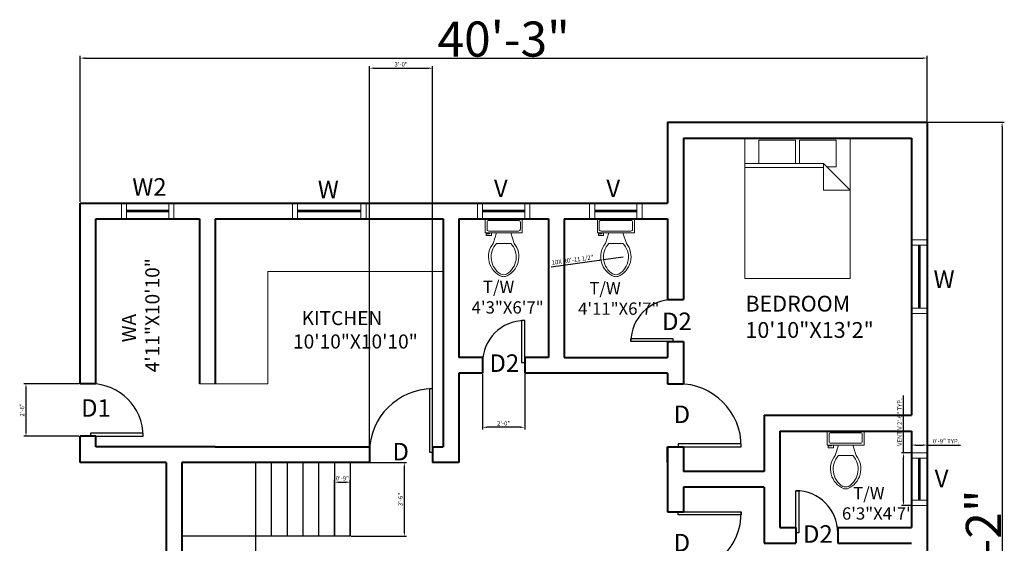
# Model space of a CAD drawing. Units: inches. Extents: x 4878 to 9282, y 5367 to 6617.
# Tile 11 of 14: x 7961 to 8522, y 6318 to 6616. Entities that reach past the tile are written whole.
import ezdxf

# ---------------------------------------------------------------- set-up
doc = ezdxf.new("R2010")
doc.units = ezdxf.units.IN
for name, color, linetype, lineweight in [('A-ANNO-DIMS', 2, 'Continuous', 18), ('A-ANNO-TEXT', 7, 'Continuous', 18), ('A-AREA-IDEN', 4, 'Continuous', 18), ('A-DOOR', 3, 'Continuous', 25), ('A-FLOR-FIXT', 9, 'Continuous', 20), ('A-FLOR-STRS', 7, 'Continuous', 25), ('A-FURN', 8, 'Continuous', 18), ('A-GLAZ', 30, 'Continuous', 20), ('A-WALL', 7, 'Continuous', 40)]:
    doc.layers.add(name, color=color, linetype=linetype, lineweight=lineweight)
doc.styles.get("Standard").update_dxf_attribs({"font": 'arial.ttf'})
doc.dimstyles.new('ISO-25', dxfattribs={"dimtxt": 2.5, "dimasz": 2.5, "dimexe": 1.25, "dimexo": 0.625, "dimtad": 1, "dimdec": 0, "dimlunit": 3, "dimtxsty": 'Standard', "dimcen": 2.5, "dimadec": 0, "dimazin": 0, "dimtfac": 1, "dimtdec": 0, "dimtmove": 0, "dimatfit": 3, "dimfxl": 1, "dimarcsym": 0})

# ---------------------------------------------------------------- blocks, each defined once
blk = doc.blocks.new('Toilet - top')
for p, q in [((9.5, -6), (9.5, -2)), ((-10, -8.5), (-8, -8.5)), ((-10, -9.5), (-10, -8.5)), ((-7, -9.5), (-10, -9.5)), ((-8, -8.5), (-8, -8)), ((-7, -8), (-7, -9.5)), ((-4, -8), (-6, -14)), ((4, -8), (6, -14)), ((4, -14), (-4, -14))]:
    blk.add_line(p, q)
blk.add_lwpolyline([(10.5, -8), (10.5, 0), (-10.5, 0), (-10.5, -8)], close=True)
for points in [[(-9.5, -2), (-9.5, -6)], [(8.5, -1), (-8.5, -1)], [(-8.5, -7), (8.5, -7)]]:
    blk.add_lwpolyline(points)
for centre, radius, start, end in [((-8.62, -1.88), 0.884, 81.8699, 188.1301), ((8.62, -1.88), 0.884, 351.8699, 98.1301), ((-8.62, -6.12), 0.884, 171.8699, 278.1301), ((8.62, -6.12), 0.884, 261.8699, 8.1301), ((3.52, -21.58), 12.17, 141.4691, 247.9714), ((4.2, -21.82), 11.33, 136.3677, 238.9468), ((-3.52, -21.58), 12.17, 292.0284, 38.5307), ((-4.2, -21.82), 11.33, 301.053, 43.6321), ((0, -27.88), 4, 245.7318, 294.2682), ((0, -29), 4, 254.8605, 285.1395)]:
    blk.add_arc(centre, radius, start, end)
blk = doc.blocks.new('Bed - Queen')
for p, q in [((0, -80.00003), (0, 0)), ((0, 0), (59.99999, 0)), ((59.99999, 0), (59.99999, -80.00003)), ((7.99999, -1.2), (28.79998, -1.2)), ((7.99999, -14.4), (7.99999, -1.2)), ((28.79998, -1.2), (28.79998, -14.4)), ((31.19999, -1.2), (51.99999, -1.2)), ((31.19999, -14.4), (31.19999, -1.2)), ((51.99999, -1.2), (51.99999, -16.4)), ((0, -14.4), (44.8, -14.4)), ((44.8, -16.8), (0, -16.8)), ((59.99999, -29.6), (44.8, -14.4)), ((44.8, -14.4), (44.8, -29.6)), ((51.99999, -16.4), (46.79936, -16.4)), ((44.8, -29.6), (59.99999, -29.6)), ((59.99999, -80.00003), (0, -80.00003))]:
    blk.add_line(p, q)
blk = doc.blocks.new('*U19')
for p, q in [((0, 0), (0, -6)), ((-36, 0), (-36, -6))]:
    blk.add_line(p, q)
blk.add_lwpolyline([(0, 0), (0, 36), (-1.75, 36), (-1.75, 0)], close=True)
blk.add_arc((0, 0), 36, 90, 180)
blk = doc.blocks.new('*U21')
for p, q in [((-24, 0), (-24, -6)), ((0, 0), (0, -6))]:
    blk.add_line(p, q)
blk.add_lwpolyline([(0, 0), (0, 24), (-1.75, 24), (-1.75, 0)], close=True)
blk.add_arc((0, 0), 24, 90, 180)
blk = doc.blocks.new('*U22')
for p, q in [((0, 0), (0, -6)), ((24, 0), (24, -6))]:
    blk.add_line(p, q)
blk.add_lwpolyline([(0, 0), (0, 24), (1.75, 24), (1.75, 0)], close=True)
blk.add_arc((0, 0), 24, 0, 90)
blk = doc.blocks.new('*U20')
for p, q in [((-36, 0), (-36, 6)), ((0, 0), (0, 6))]:
    blk.add_line(p, q)
blk.add_lwpolyline([(0, 0), (0, -36), (-1.75, -36), (-1.75, 0)], close=True)
blk.add_arc((0, 0), 36, 180, 270)
blk = doc.blocks.new('*U23')
for p, q in [((0, 0), (0, 6)), ((36, 0), (36, 6))]:
    blk.add_line(p, q)
blk.add_lwpolyline([(0, 0), (0, -36), (1.75, -36), (1.75, 0)], close=True)
blk.add_arc((0, 0), 36, 270, 360)
blk = doc.blocks.new('*U24')
for p, q in [((0, 0), (0, 6)), ((30, 0), (30, 6))]:
    blk.add_line(p, q)
blk.add_lwpolyline([(0, 0), (0, -30), (1.75, -30), (1.75, 0)], close=True)
blk.add_arc((0, 0), 30, 270, 360)
blk = doc.blocks.new('*U25')
for p, q in [((0, 0), (0, -6)), ((24, 0), (24, -6))]:
    blk.add_line(p, q)
blk.add_lwpolyline([(0, 0), (0, 24), (1.75, 24), (1.75, 0)], close=True)
blk.add_arc((0, 0), 24, 0, 90)
blk = doc.blocks.new('*D26')
at = {"layer": 'A-ANNO-DIMS', "color": 0, "lineweight": -2, "transparency": 16777216}
for p, q in [((8478.72, 6557.77), (8522.05, 6557.77)), ((8520.8, 6555.27), (8520.8, 6066.27)), ((8478.72, 6063.77), (8522.05, 6063.77))]:
    blk.add_line(p, q, dxfattribs=at)
at = {"layer": 'A-ANNO-DIMS', "color": 0, "transparency": 16777216}
for points in [[(8520.39, 6555.27), (8521.22, 6555.27), (8520.8, 6557.77)], [(8520.39, 6066.27), (8521.22, 6066.27), (8520.8, 6063.77)]]:
    blk.add_solid(points, dxfattribs=at)
at = {"layer": 'Defpoints', "color": 0, "transparency": 16777216}
for p in [(8478.1, 6557.77), (8478.1, 6063.77), (8520.8, 6063.77)]:
    blk.add_point(p, dxfattribs=at)
at = {"layer": 'A-ANNO-DIMS', "color": 0, "transparency": 16777216, "insert": (8510.14, 6310.77), "char_height": 2.5, "attachment_point": 5, "rotation": 90}
blk.add_mtext('{\\H8x;41\'-2"}', dxfattribs=at)
blk = doc.blocks.new('*D27')
at = {"layer": 'A-ANNO-DIMS', "color": 0, "lineweight": -2, "transparency": 16777216}
for p, q in [((7995.1, 6512.4), (7995.1, 6595.64)), ((7997.6, 6594.39), (8475.6, 6594.39)), ((8478.1, 6512.4), (8478.1, 6595.64))]:
    blk.add_line(p, q, dxfattribs=at)
at = {"layer": 'A-ANNO-DIMS', "color": 0, "transparency": 16777216}
for points in [[(7997.6, 6594.81), (7997.6, 6593.97), (7995.1, 6594.39)], [(8475.6, 6594.81), (8475.6, 6593.97), (8478.1, 6594.39)]]:
    blk.add_solid(points, dxfattribs=at)
at = {"layer": 'Defpoints', "color": 0, "transparency": 16777216}
for p in [(8478.1, 6594.39), (7995.1, 6511.77), (8478.1, 6511.77)]:
    blk.add_point(p, dxfattribs=at)
at = {"layer": 'A-ANNO-DIMS', "color": 0, "transparency": 16777216, "insert": (8236.6, 6605.23), "char_height": 2.5, "attachment_point": 5}
blk.add_mtext('{\\H8x;40\'-3"}', dxfattribs=at)
blk = doc.blocks.new('WINDOW-PLAN-36IN')
for p, q in [((0, 0), (0, 9)), ((3, 0), (3, 9)), ((39, 0), (39, 9)), ((42, 0), (42, 9)), ((3, 5), (39, 5)), ((3, 4.5), (39, 4.5)), ((3, 4), (39, 4))]:
    blk.add_line(p, q)
blk = doc.blocks.new('WINDOW-PLAN-24IN')
for p, q in [((9, 30), (0, 30)), ((9, 27), (0, 27)), ((4, 3), (4, 27)), ((4.5, 3), (4.5, 27)), ((5, 3), (5, 27)), ((9, 3), (0, 3)), ((9, 0), (0, 0))]:
    blk.add_line(p, q)
blk = doc.blocks.new('*D41')
at = {"layer": 'A-ANNO-DIMS', "color": 0, "lineweight": -2, "transparency": 16777216}
for p, q in [((8464.6, 6369.27), (8464.6, 6401.97)), ((8468.47, 6369.27), (8463.35, 6369.27)), ((8464.6, 6341.77), (8464.6, 6366.77)), ((8468.47, 6339.27), (8463.35, 6339.27))]:
    blk.add_line(p, q, dxfattribs=at)
at = {"layer": 'A-ANNO-DIMS', "color": 0, "transparency": 16777216}
for points in [[(8464.18, 6366.77), (8465.01, 6366.77), (8464.6, 6369.27)], [(8464.18, 6341.77), (8465.01, 6341.77), (8464.6, 6339.27)]]:
    blk.add_solid(points, dxfattribs=at)
at = {"layer": 'Defpoints', "color": 0, "transparency": 16777216}
for p in [(8464.6, 6369.27), (8469.1, 6369.27), (8469.1, 6339.27)]:
    blk.add_point(p, dxfattribs=at)
at = {"layer": 'A-ANNO-DIMS', "color": 0, "transparency": 16777216, "insert": (8462.69, 6386.87), "char_height": 2.5, "attachment_point": 5, "rotation": 90}
blk.add_mtext('VENT V 2\'-6" TYP.', dxfattribs=at)
blk = doc.blocks.new('*D42')
at = {"layer": 'A-ANNO-DIMS', "color": 0, "lineweight": -2, "transparency": 16777216}
for p, q in [((8469.1, 6369.9), (8469.1, 6375.02)), ((8471.6, 6373.77), (8475.6, 6373.77)), ((8478.1, 6369.9), (8478.1, 6375.02)), ((8478.1, 6373.77), (8497.08, 6373.77))]:
    blk.add_line(p, q, dxfattribs=at)
at = {"layer": 'A-ANNO-DIMS', "color": 0, "transparency": 16777216}
for points in [[(8471.6, 6374.19), (8471.6, 6373.35), (8469.1, 6373.77)], [(8475.6, 6374.19), (8475.6, 6373.35), (8478.1, 6373.77)]]:
    blk.add_solid(points, dxfattribs=at)
at = {"layer": 'Defpoints', "color": 0, "transparency": 16777216}
for p in [(8478.1, 6373.77), (8469.1, 6369.27), (8478.1, 6369.27)]:
    blk.add_point(p, dxfattribs=at)
at = {"layer": 'A-ANNO-DIMS', "color": 0, "transparency": 16777216, "insert": (8488.84, 6375.67), "char_height": 2.5, "attachment_point": 5}
blk.add_mtext('0\'-9" TYP.', dxfattribs=at)
blk = doc.blocks.new('*D107')
at = {"layer": 'A-ANNO-DIMS', "color": 0, "lineweight": -2, "transparency": 16777216}
for p, q in [((7994.47, 6408.77), (7963, 6408.77)), ((7964.25, 6381.27), (7964.25, 6406.27)), ((7994.47, 6378.77), (7963, 6378.77))]:
    blk.add_line(p, q, dxfattribs=at)
at = {"layer": 'A-ANNO-DIMS', "color": 0, "transparency": 16777216}
for points in [[(7963.83, 6406.27), (7964.66, 6406.27), (7964.25, 6408.77)], [(7963.83, 6381.27), (7964.66, 6381.27), (7964.25, 6378.77)]]:
    blk.add_solid(points, dxfattribs=at)
at = {"layer": 'Defpoints', "color": 0, "transparency": 16777216}
for p in [(7964.25, 6408.77), (7995.1, 6408.77), (7995.1, 6378.77)]:
    blk.add_point(p, dxfattribs=at)
at = {"layer": 'A-ANNO-DIMS', "color": 0, "transparency": 16777216, "insert": (7962.34, 6393.77), "char_height": 2.5, "attachment_point": 5, "rotation": 90}
blk.add_mtext('2\'-6"', dxfattribs=at)
blk = doc.blocks.new('*D108')
at = {"layer": 'A-ANNO-DIMS', "color": 0, "lineweight": -2, "transparency": 16777216}
for p, q in [((8160.1, 6373.4), (8160.1, 6589.87)), ((8162.6, 6588.62), (8193.6, 6588.62)), ((8196.1, 6373.4), (8196.1, 6589.87))]:
    blk.add_line(p, q, dxfattribs=at)
at = {"layer": 'A-ANNO-DIMS', "color": 0, "transparency": 16777216}
for points in [[(8162.6, 6589.04), (8162.6, 6588.2), (8160.1, 6588.62)], [(8193.6, 6589.04), (8193.6, 6588.2), (8196.1, 6588.62)]]:
    blk.add_solid(points, dxfattribs=at)
at = {"layer": 'Defpoints', "color": 0, "transparency": 16777216}
for p in [(8196.1, 6588.62), (8160.1, 6372.77), (8196.1, 6372.77)]:
    blk.add_point(p, dxfattribs=at)
at = {"layer": 'A-ANNO-DIMS', "color": 0, "transparency": 16777216, "insert": (8178.1, 6590.52), "char_height": 2.5, "attachment_point": 5}
blk.add_mtext('3\'-0"', dxfattribs=at)
blk = doc.blocks.new('*D110')
at = {"layer": 'A-ANNO-DIMS', "color": 0, "lineweight": -2, "transparency": 16777216}
for p, q in [((8224.6, 6414.15), (8224.6, 6382.67)), ((8248.6, 6414.15), (8248.6, 6382.67)), ((8246.1, 6383.92), (8227.1, 6383.92))]:
    blk.add_line(p, q, dxfattribs=at)
at = {"layer": 'A-ANNO-DIMS', "color": 0, "transparency": 16777216}
for points in [[(8227.1, 6384.34), (8227.1, 6383.5), (8224.6, 6383.92)], [(8246.1, 6384.34), (8246.1, 6383.5), (8248.6, 6383.92)]]:
    blk.add_solid(points, dxfattribs=at)
at = {"layer": 'Defpoints', "color": 0, "transparency": 16777216}
for p in [(8224.6, 6414.77), (8248.6, 6414.77), (8224.6, 6383.92)]:
    blk.add_point(p, dxfattribs=at)
at = {"layer": 'A-ANNO-DIMS', "color": 0, "transparency": 16777216, "insert": (8236.6, 6385.82), "char_height": 2.5, "attachment_point": 5}
blk.add_mtext('2\'-0"', dxfattribs=at)
blk = doc.blocks.new('*D115')
at = {"layer": 'A-ANNO-DIMS', "color": 0, "lineweight": -2, "transparency": 16777216}
for p, q in [((8149.72, 6363.77), (8181.2, 6363.77)), ((8179.95, 6361.27), (8179.95, 6324.27)), ((8149.72, 6321.77), (8181.2, 6321.77))]:
    blk.add_line(p, q, dxfattribs=at)
at = {"layer": 'A-ANNO-DIMS', "color": 0, "transparency": 16777216}
for points in [[(8179.53, 6361.27), (8180.36, 6361.27), (8179.95, 6363.77)], [(8179.53, 6324.27), (8180.36, 6324.27), (8179.95, 6321.77)]]:
    blk.add_solid(points, dxfattribs=at)
at = {"layer": 'Defpoints', "color": 0, "transparency": 16777216}
for p in [(8149.1, 6363.77), (8149.1, 6321.77), (8179.95, 6321.77)]:
    blk.add_point(p, dxfattribs=at)
at = {"layer": 'A-ANNO-DIMS', "color": 0, "transparency": 16777216, "insert": (8178.04, 6342.77), "char_height": 2.5, "attachment_point": 5, "rotation": 90}
blk.add_mtext('3\'-6"', dxfattribs=at)
blk = doc.blocks.new('*D116')
at = {"layer": 'A-ANNO-DIMS', "color": 0, "lineweight": -2, "transparency": 16777216}
for p, q in [((8140.1, 6322.4), (8140.1, 6353.87)), ((8142.6, 6352.62), (8146.6, 6352.62)), ((8149.1, 6322.4), (8149.1, 6353.87))]:
    blk.add_line(p, q, dxfattribs=at)
at = {"layer": 'A-ANNO-DIMS', "color": 0, "transparency": 16777216}
for points in [[(8142.6, 6353.04), (8142.6, 6352.2), (8140.1, 6352.62)], [(8146.6, 6353.04), (8146.6, 6352.2), (8149.1, 6352.62)]]:
    blk.add_solid(points, dxfattribs=at)
at = {"layer": 'Defpoints', "color": 0, "transparency": 16777216}
for p in [(8149.1, 6352.62), (8140.1, 6321.77), (8149.1, 6321.77)]:
    blk.add_point(p, dxfattribs=at)
at = {"layer": 'A-ANNO-DIMS', "color": 0, "transparency": 16777216, "insert": (8144.6, 6354.52), "char_height": 2.5, "attachment_point": 5}
blk.add_mtext('0\'-9"', dxfattribs=at)
blk = doc.blocks.new('*D127')
at = {"layer": 'A-ANNO-DIMS', "color": 0, "lineweight": -2, "transparency": 16777216}
for p, q in [((8263.7, 6475.41), (8291.09, 6479.11)), ((8304.8, 6480.95), (8293.57, 6479.44))]:
    blk.add_line(p, q, dxfattribs=at)
at = {"layer": 'A-ANNO-DIMS', "color": 0, "transparency": 16777216}
blk.add_solid([(8291.04, 6479.52), (8291.15, 6478.69), (8293.57, 6479.44)], dxfattribs=at)
at = {"layer": 'Defpoints', "color": 0, "transparency": 16777216}
for p in [(8293.57, 6479.44), (8304.8, 6480.95)]:
    blk.add_point(p, dxfattribs=at)
at = {"layer": 'A-ANNO-DIMS', "color": 0, "transparency": 16777216, "insert": (8275.9, 6478.99), "char_height": 2.5, "attachment_point": 5, "rotation": 7.6808}
blk.add_mtext('10X R0\'-11 1/2"', dxfattribs=at)

msp = doc.modelspace()

# ---------------------------------------------------------------- linework, layer by layer
at = {"layer": 'A-FLOR-FIXT'}
for p, q in [((8102.1, 6472.77), (8102.1, 6408.77)), ((8102.1, 6472.77), (8202.1, 6472.77)), ((8102.1, 6408.77), (8063.1, 6408.77))]:
    msp.add_line(p, q, dxfattribs=at)
at = {"layer": 'A-FLOR-STRS'}
for p, q in [((8095.1, 6363.77), (8095.1, 6222.77)), ((8104.1, 6363.77), (8104.1, 6321.77)), ((8113.1, 6363.77), (8113.1, 6321.77)), ((8122.1, 6363.77), (8122.1, 6321.77)), ((8131.1, 6363.77), (8131.1, 6321.77)), ((8140.1, 6363.77), (8140.1, 6321.77)), ((8149.1, 6363.77), (8149.1, 6321.77)), ((8149.1, 6321.77), (8053.1, 6321.77))]:
    msp.add_line(p, q, dxfattribs=at)
at = {"layer": 'A-WALL'}
for p, q in [((8330.1, 6557.77), (8330.1, 6511.77)), ((8330.1, 6557.77), (8478.1, 6557.77)), ((8478.1, 6557.77), (8478.1, 6174.77)), ((8339.1, 6548.77), (8339.1, 6456.77)), ((8339.1, 6548.77), (8469.1, 6548.77)), ((8469.1, 6548.77), (8469.1, 6390.77)), ((7995.1, 6511.77), (8330.1, 6511.77)), ((7995.1, 6408.77), (7995.1, 6511.77)), ((8072.1, 6511.77), (8202.1, 6511.77)), ((8211.1, 6511.77), (8262.1, 6511.77)), ((8271.1, 6511.77), (8330.1, 6511.77)), ((8004.1, 6502.77), (8063.1, 6502.77)), ((8004.1, 6408.77), (8004.1, 6502.77)), ((8063.1, 6502.77), (8063.1, 6408.77)), ((8072.1, 6502.77), (8072.1, 6408.77)), ((8072.1, 6502.77), (8202.1, 6502.77)), ((8202.1, 6502.77), (8202.1, 6372.77)), ((8211.1, 6502.77), (8211.1, 6423.77)), ((8211.1, 6502.77), (8262.1, 6502.77)), ((8262.1, 6502.77), (8262.1, 6423.77)), ((8271.1, 6502.77), (8271.1, 6423.77)), ((8271.1, 6502.77), (8330.1, 6502.77)), ((8330.1, 6502.77), (8330.1, 6456.77)), ((8330.1, 6456.77), (8339.1, 6456.77)), ((8330.1, 6432.77), (8339.1, 6432.77)), ((8330.1, 6432.77), (8330.1, 6423.77)), ((8339.1, 6432.77), (8339.1, 6408.77)), ((8339.1, 6432.77), (8339.1, 6408.77)), ((8224.6, 6423.77), (8211.1, 6423.77)), ((8224.6, 6423.77), (8224.6, 6414.77)), ((8262.1, 6423.77), (8248.6, 6423.77)), ((8248.6, 6423.77), (8248.6, 6414.77)), ((8271.1, 6423.77), (8330.1, 6423.77)), ((8224.6, 6414.77), (8211.1, 6414.77)), ((8211.1, 6414.77), (8211.1, 6363.77)), ((8330.1, 6414.77), (8248.6, 6414.77)), ((8330.1, 6414.77), (8330.1, 6408.77)), ((8004.1, 6408.77), (7995.1, 6408.77)), ((8330.1, 6408.77), (8339.1, 6408.77)), ((8385.1, 6390.77), (8385.1, 6358.77)), ((8385.1, 6390.77), (8469.1, 6390.77)), ((7995.1, 6363.77), (7995.1, 6378.77)), ((8004.1, 6378.77), (7995.1, 6378.77)), ((8004.1, 6372.77), (8004.1, 6378.77)), ((8394.1, 6381.77), (8394.1, 6326.77)), ((8394.1, 6381.77), (8469.1, 6381.77)), ((8469.1, 6381.77), (8469.1, 6326.77)), ((8072.1, 6372.77), (8004.1, 6372.77)), ((8072.1, 6372.77), (8160.1, 6372.77)), ((8160.1, 6372.77), (8160.1, 6363.77)), ((8196.1, 6372.77), (8196.1, 6363.77)), ((8196.1, 6372.77), (8202.1, 6372.77)), ((8330.1, 6363.77), (8330.1, 6372.77)), ((8330.1, 6372.77), (8339.1, 6372.77)), ((8330.1, 6372.77), (8330.1, 6335.77)), ((8339.1, 6372.77), (8339.1, 6363.77)), ((8339.1, 6372.77), (8339.1, 6358.77)), ((8044.1, 6363.77), (7995.1, 6363.77)), ((8044.1, 6363.77), (8044.1, 6063.77)), ((8053.1, 6363.77), (8053.1, 6222.77)), ((8160.1, 6363.77), (8053.1, 6363.77)), ((8211.1, 6363.77), (8196.1, 6363.77)), ((8385.1, 6358.77), (8339.1, 6358.77)), ((8385.1, 6349.77), (8339.1, 6349.77)), ((8339.1, 6349.77), (8339.1, 6335.77)), ((8385.1, 6349.77), (8385.1, 6317.77)), ((8330.1, 6335.77), (8339.1, 6335.77)), ((8394.1, 6326.77), (8403.1, 6326.77)), ((8403.1, 6326.77), (8403.1, 6317.77)), ((8427.1, 6326.77), (8427.1, 6317.77)), ((8427.1, 6326.77), (8469.1, 6326.77)), ((8385.1, 6317.77), (8403.1, 6317.77)), ((8427.1, 6317.77), (8469.1, 6317.77))]:
    msp.add_line(p, q, dxfattribs=at)

# ---------------------------------------------------------------- block references
at = {"layer": 'A-DOOR', "rotation": 90}
for name, p in [('*U25', (8333.1, 6432.77)), ('*U24', (8001.1, 6378.77)), ('*U23', (8336.1, 6372.77)), ('*U20', (8336.1, 6335.77))]:
    msp.add_blockref(name, p, dxfattribs=at)
at = {"layer": 'A-DOOR'}
for name, p in [('*U21', (8248.6, 6420.77)), ('*U19', (8196.1, 6369.77)), ('*U22', (8403.1, 6323.77))]:
    msp.add_blockref(name, p, dxfattribs=at)
at = {"layer": 'A-FLOR-FIXT'}
for p in [(8236.6, 6502.77), (8300.6, 6502.77), (8431.6, 6381.77)]:
    msp.add_blockref('Toilet - top', p, dxfattribs=at)
at = {"layer": 'A-FURN'}
msp.add_blockref('Bed - Queen', (8374.1, 6548.77), dxfattribs=at)
at = {"layer": 'A-GLAZ', "extrusion": (0, 0, -1), "zscale": -1, "rotation": 90}
for name, p in [('WINDOW-PLAN-24IN', (-8018.6, 6502.77)), ('WINDOW-PLAN-24IN', (-8221.6, 6502.77)), ('WINDOW-PLAN-24IN', (-8285.6, 6502.77)), ('WINDOW-PLAN-36IN', (-8469.1, 6448.77))]:
    msp.add_blockref(name, p, dxfattribs=at)
at = {"layer": 'A-GLAZ'}
for name, p in [('WINDOW-PLAN-36IN', (8116.1, 6502.77)), ('WINDOW-PLAN-24IN', (8469.1, 6339.27))]:
    msp.add_blockref(name, p, dxfattribs=at)

# ---------------------------------------------------------------- texts
at = {"layer": 'A-ANNO-TEXT', "char_height": 10, "attachment_point": 1}
for s, width, insert in [('W2', 613.0579, (8024.84, 6525.91)), ('W', 613.0579, (8130.6, 6524.52)), ('V', 613.0579, (8231.03, 6525.15)), ('V', 613.0579, (8295.15, 6525.15)), ('W', 613.0579, (8481.72, 6473.3)), ('D2', 613.0579, (8326.9, 6449.3)), ('D2', 613.0579, (8228.48, 6425.47)), ('D1', 613.0579, (7995.65, 6399.91)), ('D', 376.4819, (8333.51, 6396.32)), ('D', 376.4819, (8173.21, 6375.02)), ('V', 613.0579, (8482.34, 6359.71)), ('D2', 613.0579, (8407.26, 6328.07)), ('D', 376.4819, (8333.51, 6323.15))]:
    msp.add_mtext_dynamic_manual_height_columns(s, width=width, gutter_width=12.5, heights=[0], dxfattribs=dict(at, insert=insert))
at = {"layer": 'A-AREA-IDEN', "insert": (8018.95, 6415.25), "char_height": 8, "attachment_point": 1, "rotation": 90}
msp.add_mtext_dynamic_manual_height_columns('       WA\\P4\'11"X10\'10"', width=192.981, gutter_width=12.5, heights=[0], dxfattribs=at)
at = {"layer": 'A-AREA-IDEN', "attachment_point": 1}
for s, width, insert, char_height in [('   T/W\\P4\'3"X6\'7"', 304.9234, (8218.35, 6467.41), 7), ('   T/W\\P4\'11"X6\'7"', 304.9234, (8279.04, 6466.71), 7), ('BEDROOM\\P10\'10"X13\'2"', 268.3634, (8374.43, 6458.89), 9), ('  KITCHEN\\P10\'10"X10\'10"', 310.6043, (8116.49, 6450.16), 8), ('   T/W\\P6\'3"X4\'7"', 304.9234, (8429.49, 6349.93), 7)]:
    msp.add_mtext_dynamic_manual_height_columns(s, width=width, gutter_width=12.5, heights=[0], dxfattribs=dict(at, insert=insert, char_height=char_height))

# ---------------------------------------------------------------- dimensions: what is measured, and where the dimension line sits
at = {"layer": 'A-ANNO-DIMS'}
for base, p1, p2, text, override, picture, middle in [((8478.1, 6594.39), (7995.1, 6511.77), (8478.1, 6511.77), '{\\H8x;<>}', {"dimclrd": 0, "dimclre": 0, "dimclrt": 0}, '*D27', (8236.6, 6605.23)), ((8478.1, 6373.77), (8469.1, 6369.27), (8478.1, 6369.27), '<> TYP.', {"dimdec": 1, "dimlfac": 1, "dimrnd": 0, "dimzin": 1, "dimdsep": 46, "dimlunit": 4, "dimfrac": 2}, '*D42', (8488.84, 6375.67))]:
    dim = msp.add_linear_dim(base=base, p1=p1, p2=p2, text=text, dimstyle='ISO-25', override=override, dxfattribs=at)
    dim.commit()
    dim.dimension.update_dxf_attribs({"geometry": picture, "text_midpoint": middle})
for base, p1, p2, picture, middle in [((8196.1, 6588.62), (8160.1, 6372.77), (8196.1, 6372.77), '*D108', (8178.1, 6590.52)), ((8149.1, 6352.62), (8140.1, 6321.77), (8149.1, 6321.77), '*D116', (8144.6, 6354.52))]:
    dim = msp.add_linear_dim(base=base, p1=p1, p2=p2, dimstyle='ISO-25', override={"dimdec": 1, "dimlfac": 1, "dimrnd": 0, "dimzin": 1, "dimdsep": 46, "dimlunit": 4, "dimfrac": 2}, dxfattribs=at)
    dim.commit()
    dim.dimension.update_dxf_attribs({"geometry": picture, "text_midpoint": middle})
for base, p1, p2, text, override, picture, middle in [((8520.8, 6063.77), (8478.1, 6557.77), (8478.1, 6063.77), '{\\H8x;<>}', {"dimclrd": 0, "dimclre": 0, "dimclrt": 0}, '*D26', (8510.14, 6310.77)), ((8464.6, 6369.27), (8469.1, 6339.27), (8469.1, 6369.27), 'VENT V <> TYP.', {"dimdec": 1, "dimlfac": 1, "dimrnd": 0, "dimzin": 1, "dimdsep": 46, "dimlunit": 4, "dimfrac": 2}, '*D41', (8462.69, 6386.87))]:
    dim = msp.add_linear_dim(base=base, p1=p1, p2=p2, angle=90, text=text, dimstyle='ISO-25', override=override, dxfattribs=at)
    dim.commit()
    dim.dimension.update_dxf_attribs({"geometry": picture, "text_midpoint": middle})
dim = msp.add_radius_dim(center=(8304.8, 6480.95), mpoint=(8293.57, 6479.44), text='10X <>', dimstyle='ISO-25', override={"dimdec": 1, "dimlfac": 1, "dimrnd": 0, "dimzin": 1, "dimdsep": 46, "dimlunit": 4, "dimfrac": 2}, dxfattribs=at)
dim.commit()
dim.dimension.update_dxf_attribs({"geometry": '*D127', "text_midpoint": (8275.9, 6478.99)})
for base, p1, p2, angle, picture, middle in [((8224.6, 6383.92), (8248.6, 6414.77), (8224.6, 6414.77), 180, '*D110', (8236.6, 6385.82)), ((7964.25, 6408.77), (7995.1, 6378.77), (7995.1, 6408.77), 90, '*D107', (7962.34, 6393.77)), ((8179.95, 6321.77), (8149.1, 6363.77), (8149.1, 6321.77), 270, '*D115', (8178.04, 6342.77))]:
    dim = msp.add_linear_dim(base=base, p1=p1, p2=p2, angle=angle, dimstyle='ISO-25', override={"dimdec": 1, "dimlfac": 1, "dimrnd": 0, "dimzin": 1, "dimdsep": 46, "dimlunit": 4, "dimfrac": 2}, dxfattribs=at)
    dim.commit()
    dim.dimension.update_dxf_attribs({"geometry": picture, "text_midpoint": middle})

doc.saveas('drawing.dxf')
